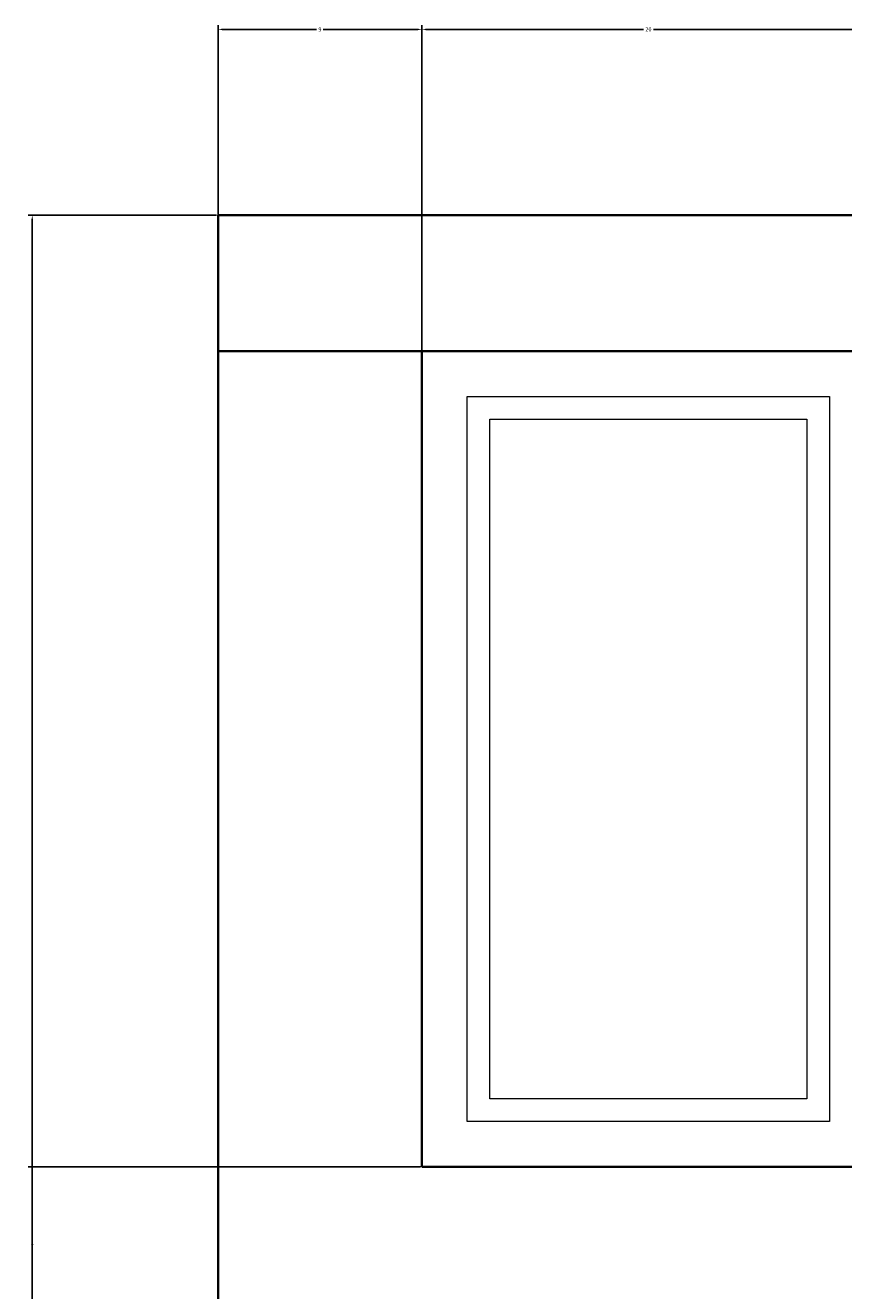
# Model space of a CAD drawing. Units: inches. Extents: x 27 to 200, y -50 to 102.
# Tile 6 of 26: x 27 to 63, y 46 to 102. Entities that reach past the tile are written whole.
import ezdxf

# ---------------------------------------------------------------- set-up
doc = ezdxf.new("R2010")
doc.units = ezdxf.units.IN
doc.header["$MEASUREMENT"] = 0
for name, color, linetype, lineweight in [('A-ANNO-DIMS', 2, 'Continuous', 18), ('A-ELEV', 7, 'Continuous', 35), ('A-FURN', 8, 'Continuous', 18)]:
    doc.layers.add(name, color=color, linetype=linetype, lineweight=lineweight)
doc.styles.get("Standard").update_dxf_attribs({"font": 'arial.ttf'})
doc.dimstyles.get("Standard").update_dxf_attribs({"dimtxt": 0.18, "dimasz": 0.18, "dimexe": 0.18, "dimexo": 0.0625, "dimgap": 0.09, "dimtad": 0, "dimtih": 1, "dimtoh": 1, "dimdec": 4, "dimzin": 0, "dimdsep": 46, "dimtxsty": 'Standard', "dimcen": 0.09, "dimadec": 0, "dimazin": 0, "dimtfac": 1, "dimtdec": 4, "dimtofl": 0, "dimtmove": 0, "dimatfit": 3, "dimfxl": 1, "dimtolj": 1, "dimtzin": 0, "dimarcsym": 0})

# ---------------------------------------------------------------- blocks, each defined once
blk = doc.blocks.new('CAB-DOOR-TALL')
for p, q in [((0, 0), (0, 32)), ((0, 32), (16, 32)), ((16, 32), (16, 0)), ((1, 1), (1, 31)), ((1, 31), (15, 31)), ((15, 31), (15, 1)), ((15, 1), (1, 1)), ((16, 0), (0, 0))]:
    blk.add_line(p, q)
blk = doc.blocks.new('*D13')
at = {"layer": 'A-ANNO-DIMS', "color": 0, "lineweight": -2, "transparency": 16777216}
for p, q in [((35.417, 87.989), (35.417, 102.306)), ((44.417, 87.989), (44.417, 102.306)), ((35.597, 102.126), (39.768, 102.126)), ((44.237, 102.126), (40.066, 102.126))]:
    blk.add_line(p, q, dxfattribs=at)
at = {"layer": 'A-ANNO-DIMS', "color": 0, "transparency": 16777216}
for points in [[(35.597, 102.156), (35.597, 102.096), (35.417, 102.126)], [(44.237, 102.156), (44.237, 102.096), (44.417, 102.126)]]:
    blk.add_solid(points, dxfattribs=at)
at = {"layer": 'Defpoints', "color": 0, "transparency": 16777216}
for p in [(44.417, 102.126), (35.417, 87.926), (44.417, 87.926)]:
    blk.add_point(p, dxfattribs=at)
at = {"layer": 'A-ANNO-DIMS', "color": 0, "transparency": 16777216, "insert": (39.917, 102.126), "char_height": 0.18, "attachment_point": 5}
blk.add_mtext('\\A1;9', dxfattribs=at)
blk = doc.blocks.new('*D14')
at = {"layer": 'A-ANNO-DIMS', "color": 0, "lineweight": -2, "transparency": 16777216}
for p, q in [((44.417, 87.989), (44.417, 102.306)), ((64.417, 87.989), (64.417, 102.306)), ((44.597, 102.126), (54.197, 102.126)), ((64.237, 102.126), (54.637, 102.126))]:
    blk.add_line(p, q, dxfattribs=at)
at = {"layer": 'A-ANNO-DIMS', "color": 0, "transparency": 16777216}
for points in [[(44.597, 102.156), (44.597, 102.096), (44.417, 102.126)], [(64.237, 102.156), (64.237, 102.096), (64.417, 102.126)]]:
    blk.add_solid(points, dxfattribs=at)
at = {"layer": 'Defpoints', "color": 0, "transparency": 16777216}
for p in [(64.417, 102.126), (44.417, 87.926), (64.417, 87.926)]:
    blk.add_point(p, dxfattribs=at)
at = {"layer": 'A-ANNO-DIMS', "color": 0, "transparency": 16777216, "insert": (54.417, 102.126), "char_height": 0.18, "attachment_point": 5}
blk.add_mtext('\\A1;20', dxfattribs=at)
blk = doc.blocks.new('*D24')
at = {"layer": 'A-ANNO-DIMS', "color": 0, "lineweight": -2, "transparency": 16777216}
for p, q in [((35.354, 93.926), (27.037, 93.926)), ((27.217, 93.746), (27.217, 38.76)), ((27.217, -16.589), (27.217, 38.397)), ((35.354, -16.769), (27.037, -16.769))]:
    blk.add_line(p, q, dxfattribs=at)
at = {"layer": 'A-ANNO-DIMS', "color": 0, "transparency": 16777216}
for points in [[(27.187, 93.746), (27.247, 93.746), (27.217, 93.926)], [(27.187, -16.589), (27.247, -16.589), (27.217, -16.769)]]:
    blk.add_solid(points, dxfattribs=at)
at = {"layer": 'Defpoints', "color": 0, "transparency": 16777216}
for p in [(27.217, 93.926), (35.417, 93.926), (35.417, -16.769)]:
    blk.add_point(p, dxfattribs=at)
at = {"layer": 'A-ANNO-DIMS', "color": 0, "transparency": 16777216, "insert": (27.217, 38.579), "char_height": 0.18, "attachment_point": 5}
blk.add_mtext('\\A1;110.7', dxfattribs=at)
blk = doc.blocks.new('*D47')
at = {"layer": 'A-ANNO-DIMS', "color": 0, "lineweight": -2, "transparency": 16777216}
for p, q in [((44.354402, 51.926437), (27.036902, 51.926437)), ((27.216902, 51.746437), (27.216902, 48.606437)), ((27.216902, 45.106437), (27.216902, 48.246437)), ((44.354402, 44.926437), (27.036902, 44.926437))]:
    blk.add_line(p, q, dxfattribs=at)
at = {"layer": 'A-ANNO-DIMS', "color": 0, "transparency": 16777216}
for points in [[(27.186902, 51.746437), (27.246902, 51.746437), (27.216902, 51.926437)], [(27.186902, 45.106437), (27.246902, 45.106437), (27.216902, 44.926437)]]:
    blk.add_solid(points, dxfattribs=at)
at = {"layer": 'Defpoints', "color": 0, "transparency": 16777216}
for p in [(27.216902, 51.926437), (44.416902, 51.926437), (44.416902, 44.926437)]:
    blk.add_point(p, dxfattribs=at)
at = {"layer": 'A-ANNO-DIMS', "color": 0, "transparency": 16777216, "insert": (27.216902, 48.426437), "char_height": 0.18, "attachment_point": 5}
blk.add_mtext('\\A1;7', dxfattribs=at)

msp = doc.modelspace()

# ---------------------------------------------------------------- linework, layer by layer
at = {"layer": 'A-ELEV'}
for p, q in [((191.4169, 93.9264), (35.4169, 93.9264)), ((35.4169, 93.9264), (35.4169, -16.7693)), ((191.4169, 87.9264), (35.4169, 87.9264)), ((44.4169, 51.9264), (44.4169, 87.9264)), ((84.4169, 51.9264), (44.4169, 51.9264))]:
    msp.add_line(p, q, dxfattribs=at)

# ---------------------------------------------------------------- block references
at = {"layer": 'A-FURN'}
msp.add_blockref('CAB-DOOR-TALL', (46.417, 53.926), dxfattribs=at)

# ---------------------------------------------------------------- dimensions: what is measured, and where the dimension line sits
at = {"layer": 'A-ANNO-DIMS'}
for base, p1, p2, picture, middle in [((44.4169, 102.1264), (35.4169, 87.9264), (44.4169, 87.9264), '*D13', (39.9169, 102.1264)), ((64.4169, 102.1264), (44.4169, 87.9264), (64.4169, 87.9264), '*D14', (54.4169, 102.1264))]:
    dim = msp.add_linear_dim(base=base, p1=p1, p2=p2, dimstyle='Standard', override={"dimdec": 0, "dimlfac": 1, "dimrnd": 0, "dimzin": 0, "dimdsep": 46, "dimlunit": 2}, dxfattribs=at)
    dim.commit()
    dim.dimension.update_dxf_attribs({"geometry": picture, "text_midpoint": middle})
for base, p1, p2, override, picture, middle in [((27.2169, 93.9264), (35.4169, -16.7693), (35.4169, 93.9264), {"dimdec": 1, "dimlfac": 1, "dimrnd": 0, "dimzin": 0, "dimdsep": 46, "dimlunit": 2}, '*D24', (27.2169, 38.5786)), ((27.2169, 51.9264), (44.4169, 44.9264), (44.4169, 51.9264), {"dimdec": 0, "dimlfac": 1, "dimrnd": 0, "dimzin": 0, "dimdsep": 46, "dimlunit": 2}, '*D47', (27.2169, 48.4264))]:
    dim = msp.add_linear_dim(base=base, p1=p1, p2=p2, angle=90, dimstyle='Standard', override=override, dxfattribs=at)
    dim.commit()
    dim.dimension.update_dxf_attribs({"geometry": picture, "text_midpoint": middle})

doc.saveas('drawing.dxf')
